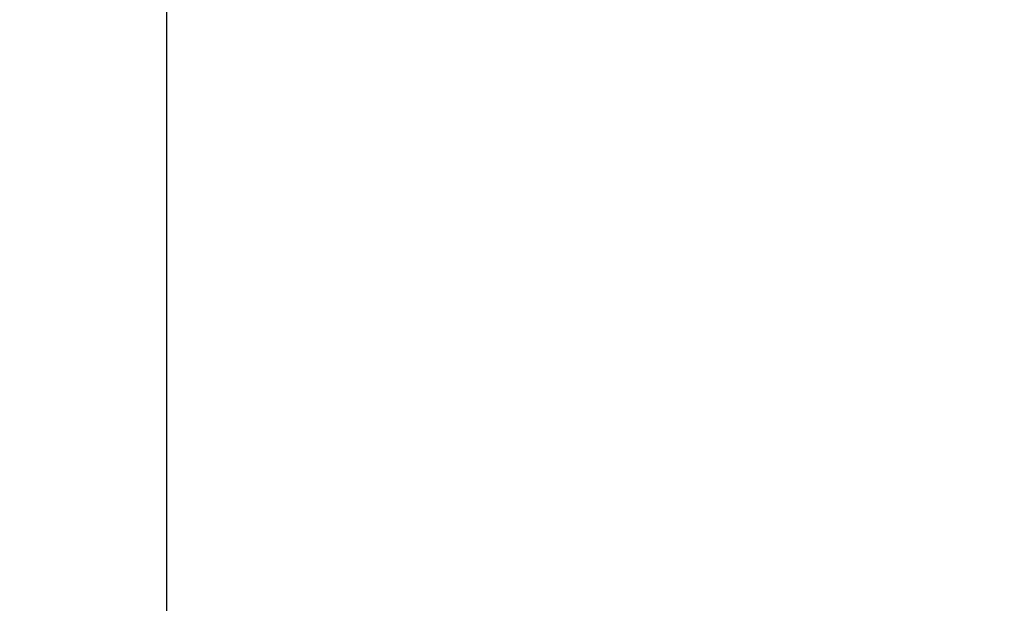
# Model space of a CAD drawing. Units: inches. Extents: x -48 to 50072, y 0 to 21068.
# Tile 17 of 75: x 289 to 341, y 278 to 309. Entities that reach past the tile are written whole.
import ezdxf

# ---------------------------------------------------------------- set-up
doc = ezdxf.new("R2010")
doc.units = ezdxf.units.IN
doc.header["$MEASUREMENT"] = 0
doc.layers.add('A-ANNO-DIMS', color=2, linetype='Continuous', lineweight=18)
doc.styles.get("Standard").update_dxf_attribs({"font": 'arial.ttf'})
doc.dimstyles.get("Standard").update_dxf_attribs({"dimtxt": 8, "dimasz": 0.18, "dimexe": 0.18, "dimexo": 0.0625, "dimgap": 0.09, "dimtad": 0, "dimtih": 1, "dimtoh": 1, "dimdec": 1, "dimzin": 0, "dimdsep": 46, "dimlunit": 4, "dimtxsty": 'Standard', "dimblk": 'ARCHTICK', "dimcen": 0.09, "dimadec": 0, "dimazin": 0, "dimtfac": 1, "dimtdec": 1, "dimtofl": 0, "dimtmove": 0, "dimatfit": 3, "dimldrblk": 'ARCHTICK', "dimfxl": 1, "dimtolj": 1, "dimtzin": 0, "dimarcsym": 0})

# ---------------------------------------------------------------- blocks, each defined once
blk = doc.blocks.new('_ArchTick')
at = {"color": 0, "linetype": 'ByBlock', "const_width": 0.15}
blk.add_lwpolyline([(-0.5, -0.5), (0.5, 0.5)], dxfattribs=at)
blk = doc.blocks.new('*D117')
at = {"layer": 'A-ANNO-DIMS', "color": 0, "lineweight": -2, "transparency": 16777216}
for p, q in [((216.017, 488.712), (216.017, 165.945)), ((297.017, 488.712), (297.017, 165.945)), ((216.017, 166.125), (251.464, 166.125)), ((297.017, 166.125), (261.57, 166.125))]:
    blk.add_line(p, q, dxfattribs=at)
at = {"layer": 'Defpoints', "color": 0, "transparency": 16777216}
for p in [(216.017, 488.775), (297.017, 488.775), (297.017, 166.125)]:
    blk.add_point(p, dxfattribs=at)
at = {"layer": 'A-ANNO-DIMS', "color": 0, "lineweight": -2, "transparency": 16777216, "xscale": 0.18, "yscale": 0.18, "zscale": 0.18, "rotation": 180}
blk.add_blockref('_ArchTick', (216.017, 166.125), dxfattribs=at)
at = {"layer": 'A-ANNO-DIMS', "color": 0, "lineweight": -2, "transparency": 16777216, "xscale": 0.18, "yscale": 0.18, "zscale": 0.18}
blk.add_blockref('_ArchTick', (297.017, 166.125), dxfattribs=at)
at = {"layer": 'A-ANNO-DIMS', "color": 0, "transparency": 16777216, "insert": (256.517, 166.125), "char_height": 8, "attachment_point": 5}
blk.add_mtext('\\A1;81', dxfattribs=at)
blk = doc.blocks.new('*D118')
at = {"layer": 'A-ANNO-DIMS', "color": 0, "lineweight": -2, "transparency": 16777216}
for p, q in [((297.017, 488.712), (297.017, 165.945)), ((463.517, 488.712), (463.517, 165.945)), ((297.017, 166.125), (367.026, 166.125)), ((463.517, 166.125), (393.509, 166.125))]:
    blk.add_line(p, q, dxfattribs=at)
at = {"layer": 'Defpoints', "color": 0, "transparency": 16777216}
for p in [(297.017, 488.775), (463.517, 488.775), (463.517, 166.125)]:
    blk.add_point(p, dxfattribs=at)
at = {"layer": 'A-ANNO-DIMS', "color": 0, "lineweight": -2, "transparency": 16777216, "xscale": 0.18, "yscale": 0.18, "zscale": 0.18, "rotation": 180}
blk.add_blockref('_ArchTick', (297.017, 166.125), dxfattribs=at)
at = {"layer": 'A-ANNO-DIMS', "color": 0, "lineweight": -2, "transparency": 16777216, "xscale": 0.18, "yscale": 0.18, "zscale": 0.18}
blk.add_blockref('_ArchTick', (463.517, 166.125), dxfattribs=at)
at = {"layer": 'A-ANNO-DIMS', "color": 0, "transparency": 16777216, "insert": (380.267, 166.125), "char_height": 8, "attachment_point": 5}
blk.add_mtext('\\A1;166.5', dxfattribs=at)

msp = doc.modelspace()

# ---------------------------------------------------------------- dimensions: what is measured, and where the dimension line sits
at = {"layer": 'A-ANNO-DIMS'}
for base, p1, p2, override, picture, middle in [((297.017, 166.125), (216.017, 488.775), (297.017, 488.775), {"dimdec": 0, "dimlfac": 1, "dimrnd": 0, "dimzin": 0, "dimdsep": 46, "dimlunit": 2}, '*D117', (256.517, 166.125)), ((463.517, 166.125), (297.017, 488.775), (463.517, 488.775), {"dimdec": 1, "dimlfac": 1, "dimrnd": 0, "dimzin": 0, "dimdsep": 46, "dimlunit": 2}, '*D118', (380.267, 166.125))]:
    dim = msp.add_linear_dim(base=base, p1=p1, p2=p2, dimstyle='Standard', override=override, dxfattribs=at)
    dim.commit()
    dim.dimension.update_dxf_attribs({"geometry": picture, "text_midpoint": middle})

doc.saveas('drawing.dxf')
